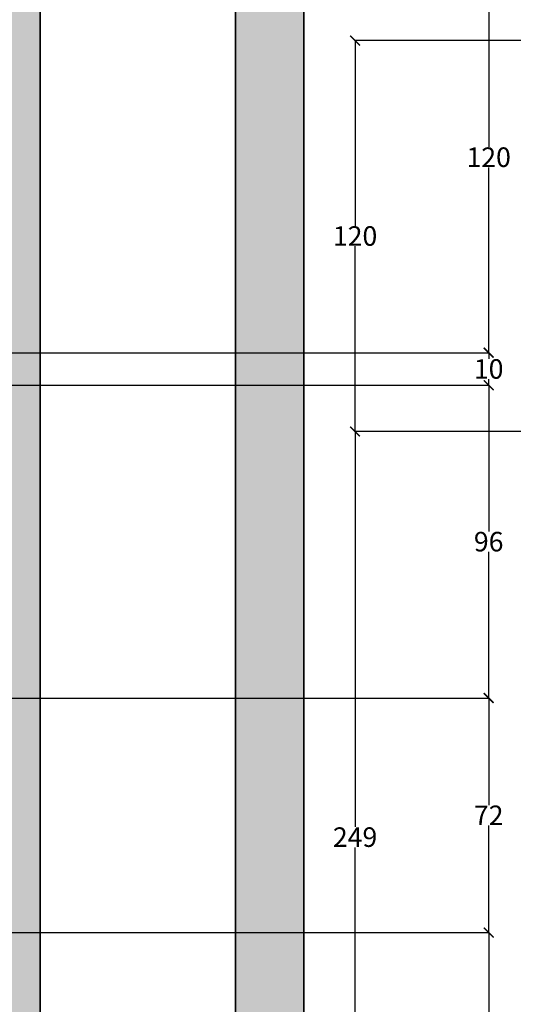
# Model space of a CAD drawing. Units: inches. Extents: x 925 to 2834, y 111 to 1355.
# Tile 22 of 25: x 1844 to 1996, y 882 to 1184. Entities that reach past the tile are written whole.
import ezdxf

# ---------------------------------------------------------------- set-up
doc = ezdxf.new("R2010")
doc.units = ezdxf.units.IN
doc.header["$MEASUREMENT"] = 0
for name, color, linetype, lineweight in [('A-ANNO-DIMS', 2, 'Continuous', 18), ('A-ANNO-TTLB', 7, 'Continuous', 35), ('A-FLOR-PATT', 252, 'Continuous', 13)]:
    doc.layers.add(name, color=color, linetype=linetype, lineweight=lineweight)
doc.styles.get("Standard").update_dxf_attribs({"font": 'arial.ttf'})
doc.dimstyles.get("Standard").update_dxf_attribs({"dimtxt": 6, "dimasz": 3, "dimexe": 0.18, "dimexo": 0.0625, "dimgap": 0.09, "dimtad": 0, "dimtih": 1, "dimtoh": 1, "dimdec": 1, "dimzin": 0, "dimdsep": 46, "dimlunit": 3, "dimtxsty": 'Standard', "dimblk": 'ARCHTICK', "dimcen": 0.09, "dimadec": 0, "dimazin": 0, "dimtfac": 1, "dimtdec": 1, "dimtofl": 0, "dimtmove": 0, "dimatfit": 3, "dimfxl": 1, "dimtolj": 1, "dimtzin": 0, "dimarcsym": 0})

# ---------------------------------------------------------------- blocks, each defined once
blk = doc.blocks.new('_ArchTick')
at = {"color": 0, "linetype": 'ByBlock', "const_width": 0.15}
blk.add_lwpolyline([(-0.5, -0.5), (0.5, 0.5)], dxfattribs=at)
blk = doc.blocks.new('*D47')
at = {"layer": 'A-ANNO-DIMS', "color": 0, "lineweight": -2, "transparency": 16777216}
for p, q in [((1708.78, 903.59), (1988.62, 903.59)), ((1988.44, 903.59), (1988.44, 869.23)), ((1988.44, 828.59), (1988.44, 862.95)), ((1708.78, 828.59), (1988.62, 828.59))]:
    blk.add_line(p, q, dxfattribs=at)
at = {"layer": 'Defpoints', "color": 0, "transparency": 16777216}
for p in [(1708.71, 903.59), (1988.44, 903.59), (1708.71, 828.59)]:
    blk.add_point(p, dxfattribs=at)
at = {"layer": 'A-ANNO-DIMS', "color": 0, "lineweight": -2, "transparency": 16777216, "xscale": 3, "yscale": 3, "zscale": 3}
for p, rotation in [((1988.44, 903.59), 90), ((1988.44, 828.59), 270)]:
    blk.add_blockref('_ArchTick', p, dxfattribs=dict(at, rotation=rotation))
at = {"layer": 'A-ANNO-DIMS', "color": 0, "transparency": 16777216, "insert": (1988.44, 866.09), "char_height": 6, "attachment_point": 5}
blk.add_mtext('\\A1;75', dxfattribs=at)
blk = doc.blocks.new('*D48')
at = {"layer": 'A-ANNO-DIMS', "color": 0, "lineweight": -2, "transparency": 16777216}
for p, q in [((1708.78, 975.59), (1988.62, 975.59)), ((1988.44, 975.59), (1988.44, 942.69)), ((1988.44, 903.59), (1988.44, 936.49)), ((1708.78, 903.59), (1988.62, 903.59))]:
    blk.add_line(p, q, dxfattribs=at)
at = {"layer": 'Defpoints', "color": 0, "transparency": 16777216}
for p in [(1708.71, 975.59), (1988.44, 975.59), (1708.71, 903.59)]:
    blk.add_point(p, dxfattribs=at)
at = {"layer": 'A-ANNO-DIMS', "color": 0, "lineweight": -2, "transparency": 16777216, "xscale": 3, "yscale": 3, "zscale": 3}
for p, rotation in [((1988.44, 975.59), 90), ((1988.44, 903.59), 270)]:
    blk.add_blockref('_ArchTick', p, dxfattribs=dict(at, rotation=rotation))
at = {"layer": 'A-ANNO-DIMS', "color": 0, "transparency": 16777216, "insert": (1988.44, 939.59), "char_height": 6, "attachment_point": 5}
blk.add_mtext('\\A1;72', dxfattribs=at)
blk = doc.blocks.new('*D49')
at = {"layer": 'A-ANNO-DIMS', "color": 0, "lineweight": -2, "transparency": 16777216}
for p, q in [((1708.78, 1071.59), (1988.62, 1071.59)), ((1988.44, 1071.59), (1988.44, 1026.74)), ((1988.44, 975.59), (1988.44, 1020.44)), ((1708.78, 975.59), (1988.62, 975.59))]:
    blk.add_line(p, q, dxfattribs=at)
at = {"layer": 'Defpoints', "color": 0, "transparency": 16777216}
for p in [(1708.71, 1071.59), (1988.44, 1071.59), (1708.71, 975.59)]:
    blk.add_point(p, dxfattribs=at)
at = {"layer": 'A-ANNO-DIMS', "color": 0, "lineweight": -2, "transparency": 16777216, "xscale": 3, "yscale": 3, "zscale": 3}
for p, rotation in [((1988.44, 1071.59), 90), ((1988.44, 975.59), 270)]:
    blk.add_blockref('_ArchTick', p, dxfattribs=dict(at, rotation=rotation))
at = {"layer": 'A-ANNO-DIMS', "color": 0, "transparency": 16777216, "insert": (1988.44, 1023.59), "char_height": 6, "attachment_point": 5}
blk.add_mtext('\\A1;96', dxfattribs=at)
blk = doc.blocks.new('*D50')
at = {"layer": 'A-ANNO-DIMS', "color": 0, "lineweight": -2, "transparency": 16777216}
for p, q in [((1718.78, 1081.59), (1988.62, 1081.59)), ((1988.44, 1081.59), (1988.44, 1079.74)), ((1988.44, 1071.59), (1988.44, 1073.44)), ((1708.78, 1071.59), (1988.62, 1071.59))]:
    blk.add_line(p, q, dxfattribs=at)
at = {"layer": 'Defpoints', "color": 0, "transparency": 16777216}
for p in [(1718.71, 1081.59), (1988.44, 1081.59), (1708.71, 1071.59)]:
    blk.add_point(p, dxfattribs=at)
at = {"layer": 'A-ANNO-DIMS', "color": 0, "lineweight": -2, "transparency": 16777216, "xscale": 3, "yscale": 3, "zscale": 3}
for p, rotation in [((1988.44, 1081.59), 90), ((1988.44, 1071.59), 270)]:
    blk.add_blockref('_ArchTick', p, dxfattribs=dict(at, rotation=rotation))
at = {"layer": 'A-ANNO-DIMS', "color": 0, "transparency": 16777216, "insert": (1988.44, 1076.59), "char_height": 6, "attachment_point": 5}
blk.add_mtext('\\A1;10', dxfattribs=at)
blk = doc.blocks.new('*D51')
at = {"layer": 'A-ANNO-DIMS', "color": 0, "lineweight": -2, "transparency": 16777216}
for p, q in [((1838.78, 1201.59), (1988.62, 1201.59)), ((1988.44, 1201.59), (1988.44, 1144.74)), ((1988.44, 1081.59), (1988.44, 1138.44)), ((1718.78, 1081.59), (1988.62, 1081.59))]:
    blk.add_line(p, q, dxfattribs=at)
at = {"layer": 'Defpoints', "color": 0, "transparency": 16777216}
for p in [(1838.71, 1201.59), (1988.44, 1201.59), (1718.71, 1081.59)]:
    blk.add_point(p, dxfattribs=at)
at = {"layer": 'A-ANNO-DIMS', "color": 0, "lineweight": -2, "transparency": 16777216, "xscale": 3, "yscale": 3, "zscale": 3}
for p, rotation in [((1988.44, 1201.59), 90), ((1988.44, 1081.59), 270)]:
    blk.add_blockref('_ArchTick', p, dxfattribs=dict(at, rotation=rotation))
at = {"layer": 'A-ANNO-DIMS', "color": 0, "transparency": 16777216, "insert": (1988.44, 1141.59), "char_height": 6, "attachment_point": 5}
blk.add_mtext('\\A1;120', dxfattribs=at)
blk = doc.blocks.new('*D79')
at = {"layer": 'A-ANNO-DIMS', "color": 0, "lineweight": -2, "transparency": 16777216}
for p, q in [((2143.61, 1057.4), (1947.23, 1057.4)), ((1947.41, 1057.4), (1947.41, 936.05)), ((1947.41, 808.4), (1947.41, 929.74)), ((2124.2, 808.4), (1947.23, 808.4))]:
    blk.add_line(p, q, dxfattribs=at)
at = {"layer": 'Defpoints', "color": 0, "transparency": 16777216}
for p in [(1947.41, 1057.4), (2143.68, 1057.4), (2124.26, 808.4)]:
    blk.add_point(p, dxfattribs=at)
at = {"layer": 'A-ANNO-DIMS', "color": 0, "lineweight": -2, "transparency": 16777216, "xscale": 3, "yscale": 3, "zscale": 3}
for p, rotation in [((1947.41, 1057.4), 90), ((1947.41, 808.4), 270)]:
    blk.add_blockref('_ArchTick', p, dxfattribs=dict(at, rotation=rotation))
at = {"layer": 'A-ANNO-DIMS', "color": 0, "transparency": 16777216, "insert": (1947.41, 932.9), "char_height": 6, "attachment_point": 5}
blk.add_mtext('\\A1;249', dxfattribs=at)
blk = doc.blocks.new('*D80')
at = {"layer": 'A-ANNO-DIMS', "color": 0, "lineweight": -2, "transparency": 16777216}
for p, q in [((2008.7, 1177.4), (1947.23, 1177.4)), ((1947.41, 1177.4), (1947.41, 1120.55)), ((1947.41, 1057.4), (1947.41, 1114.24)), ((2143.61, 1057.4), (1947.23, 1057.4))]:
    blk.add_line(p, q, dxfattribs=at)
at = {"layer": 'Defpoints', "color": 0, "transparency": 16777216}
for p in [(1947.41, 1177.4), (2008.76, 1177.4), (2143.68, 1057.4)]:
    blk.add_point(p, dxfattribs=at)
at = {"layer": 'A-ANNO-DIMS', "color": 0, "lineweight": -2, "transparency": 16777216, "xscale": 3, "yscale": 3, "zscale": 3}
for p, rotation in [((1947.41, 1177.4), 90), ((1947.41, 1057.4), 270)]:
    blk.add_blockref('_ArchTick', p, dxfattribs=dict(at, rotation=rotation))
at = {"layer": 'A-ANNO-DIMS', "color": 0, "transparency": 16777216, "insert": (1947.41, 1117.4), "char_height": 6, "attachment_point": 5}
blk.add_mtext('\\A1;120', dxfattribs=at)

msp = doc.modelspace()

# ---------------------------------------------------------------- hatches: boundary and pattern name
at = {"layer": 'A-FLOR-PATT', "transparency": 33554605}
h = msp.add_hatch(color=256, dxfattribs=at)
h.dxf.hatch_style = 1
h.paths.add_polyline_path([(1931.688, 1294.5638), (991.7375, 1294.5638), (991.7375, 172.1134), (1931.688, 172.1134)])
h.paths.add_polyline_path([(1910.7128, 1273.5886), (1910.7128, 193.0886), (1012.7128, 193.0886), (1012.7128, 1273.5886)], flags=16)
h.paths.add_polyline_path([(1850.7128, 1213.5886), (1850.7128, 253.0886), (1072.7128, 253.0886), (1072.7128, 1213.5886)], flags=0)
h.paths.add_polyline_path([(1838.7128, 1201.5886), (1838.7128, 265.0886), (1084.7128, 265.0886), (1084.7128, 530.5886), (1084.7128, 1201.5886)], flags=0)
h.paths.add_polyline_path([(1547.6758, 1155.7396), (1547.6758, 1119.115), (1513.0687, 1119.115), (1513.0687, 1155.7396)], flags=0)
h.paths.add_polyline_path([(1600.1067, 1154.9439), (1634.7139, 1154.9439), (1634.7139, 1119.115), (1600.1067, 1119.115)], flags=0)
h.paths.add_polyline_path([(1505.2502, 1144.5358), (1505.2502, 1119.115), (1470.643, 1119.115), (1470.643, 1144.5358)], flags=0)
h.paths.add_polyline_path([(1559.1357, 1141.0962), (1593.7428, 1141.0962), (1593.7428, 1119.115), (1559.1357, 1119.115)], flags=0)
h.paths.add_polyline_path([(1462.8966, 1154.9439), (1462.8966, 1119.115), (1428.2895, 1119.115), (1428.2895, 1154.9439)], flags=0)
h.paths.add_polyline_path([(1642.4603, 1144.5358), (1677.0675, 1144.5358), (1677.0675, 1119.115), (1642.4603, 1119.115)], flags=0)
h.paths.add_polyline_path([(1422.3508, 1141.0962), (1422.3508, 1119.115), (1387.7436, 1119.115), (1387.7436, 1141.0962)], flags=0)
h.paths.add_polyline_path([(1684.8859, 1155.7396), (1719.4931, 1155.7396), (1719.4931, 1119.115), (1684.8859, 1119.115)], flags=0)
h.paths.add_polyline_path([(1718.7128, 1081.5886), (1718.7128, 1050.1249), (1715.7128, 1050.1249), (1715.7128, 1026.1249), (1715.7128, 1002.1249), (1718.7128, 1002.1249), (1730.7128, 1002.1249), (1730.7128, 998.1249), (1730.7128, 990.1249), (1730.7128, 986.1249), (1718.7128, 986.1249), (1718.7128, 893.5886), (1715.3735, 893.5886), (1715.3735, 891.5886), (1713.3735, 891.5886, 0.41421356), (1677.3735, 855.5886), (1713.3735, 855.5886), (1713.3735, 853.5886), (1715.3735, 853.5886), (1715.3735, 851.5886), (1718.7128, 851.5886), (1718.7128, 821.5865), (1734.4655, 821.5865), (1734.3735, 819.5886, -0.41421356), (1712.4415, 793.5886), (1712.4415, 791.5886), (1718.7128, 791.5886), (1718.7128, 717.5886), (1718.7128, 669.5886), (1732.7128, 669.5886), (1732.7128, 665.5886), (1732.7128, 641.5886), (1732.7128, 634.5886), (1732.7128, 610.5886), (1732.7128, 603.5886), (1718.7128, 603.5886), (1718.7128, 385.0886), (1434.2128, 385.0886), (1434.2128, 530.5886), (1410.2128, 530.5886), (1408.2128, 530.5886), (1408.2128, 532.5886, 0.41421356), (1372.2128, 568.5886), (1372.2128, 532.5886), (1370.2128, 532.5886), (1370.2128, 530.5886), (1368.2128, 530.5886), (1282.2128, 530.5886), (1210.2128, 530.5886), (1200.2128, 530.5886), (1200.2128, 542.1915), (1183.2307, 542.1915), (1183.2307, 546.1915), (1200.2128, 546.1915), (1200.2128, 572.1915), (1183.2307, 572.1915), (1183.2307, 576.1915), (1200.2128, 576.1915), (1200.2128, 727.5886), (1210.2128, 727.5886), (1234.2128, 727.5886), (1259.7128, 727.5886), (1259.7128, 775.5886), (1259.7128, 799.5886), (1259.7128, 847.5886), (1259.7128, 993.5872), (1259.7128, 1065.5872), (1259.7128, 1071.5886), (1219.6318, 1071.5886), (1219.6318, 1081.5886), (1084.7128, 1081.5886), (1084.7128, 1119.115), (1256.8974, 1119.115), (1256.8974, 1154.9439), (1291.5046, 1154.9439), (1291.5046, 1119.115), (1256.8974, 1119.115), (1256.6723, 1081.5886), (1293.7128, 1081.5886), (1341.7128, 1081.5886), (1341.7128, 1093.5886), (1347.7128, 1093.5886), (1371.7128, 1093.5886), (1377.7128, 1093.5886), (1377.7128, 1081.5886), (1668.7128, 1081.5886), (1668.7128, 1117.5886), (1675.7128, 1117.5886), (1711.7128, 1117.5886), (1718.7128, 1117.5886)], flags=0)
h.paths.add_polyline_path([(1376.2838, 1155.7396), (1376.2838, 1119.115), (1341.6766, 1119.115), (1341.6766, 1155.7396)], flags=0)
h.paths.add_polyline_path([(1341.7128, 1076.0886), (1293.7128, 1076.0886), (1293.7128, 1071.5886), (1269.7128, 1071.5886), (1269.7128, 1065.5872), (1266.7128, 1065.5872), (1266.7128, 1029.5872), (1265.7128, 1029.5872), (1265.7128, 993.5872), (1269.7128, 993.5872), (1269.7128, 903.5886), (1269.7128, 893.5886), (1269.7128, 847.5886), (1265.2128, 847.5886), (1265.2128, 799.5886), (1269.7128, 799.5886), (1269.7128, 775.5886), (1265.2128, 775.5886), (1265.2128, 727.5886), (1269.7128, 727.5886), (1444.2128, 727.5886), (1444.2128, 717.5886), (1234.2128, 717.5886), (1234.2128, 722.0886), (1210.2128, 722.0886), (1210.2128, 717.5886), (1210.2128, 540.5886), (1210.2128, 536.0886), (1282.2128, 536.0886), (1282.2128, 535.0886), (1210.2128, 535.0886), (1210.2128, 540.5886), (1210.2128, 717.5886), (1210.2128, 723.0886), (1234.2128, 723.0886), (1234.2128, 717.5886), (1444.2128, 717.5886), (1444.2128, 727.5886), (1269.7128, 727.5886), (1264.2128, 727.5886), (1264.2128, 775.5886), (1269.7128, 775.5886), (1269.7128, 799.5886), (1264.2128, 799.5886), (1264.2128, 847.5886), (1269.7128, 847.5886), (1269.7128, 893.5886), (1269.7128, 903.5886), (1269.7128, 993.5872), (1264.7128, 993.5872), (1264.7128, 1029.5872), (1265.7128, 1029.5872), (1265.7128, 1065.5872), (1269.7128, 1065.5872), (1269.7128, 1071.5886), (1293.7128, 1071.5886), (1293.7128, 1077.0886), (1341.7128, 1077.0886)], flags=0)
h.paths.add_polyline_path([(1730.9529, 1141.0962), (1765.5601, 1141.0962), (1765.5601, 1119.115), (1730.9529, 1119.115)], flags=0)
h.paths.add_polyline_path([(1333.8582, 1144.5358), (1333.8582, 1119.115), (1299.251, 1119.115), (1299.251, 1144.5358)], flags=0)
h.paths.add_polyline_path([(1592.7128, 968.5886), (1596.0342, 968.5886), (1602.7128, 968.5886), (1708.7128, 968.5886), (1708.7128, 903.5886), (1602.7128, 903.5886), (1602.7128, 938.5886), (1592.7128, 938.5886), (1592.7128, 903.5886), (1451.7128, 903.5886), (1451.7128, 893.5886), (1511.7128, 893.5886), (1511.7128, 881.5886), (1515.2128, 881.5886), (1518.7128, 881.5886), (1518.7128, 893.5886), (1592.7128, 893.5886), (1592.7128, 799.5886), (1518.7128, 799.5886), (1518.7128, 857.5886), (1511.7128, 857.5886), (1511.7128, 799.5886), (1511.7128, 772.0886), (1521.7128, 772.0886), (1521.7128, 792.5886), (1592.7128, 792.5886), (1592.7128, 727.5886), (1521.7128, 727.5886), (1521.7128, 748.0886), (1511.7128, 748.0886), (1511.7128, 717.5886), (1708.7128, 717.5886), (1714.2128, 717.5886), (1714.2128, 669.5886), (1708.7128, 669.5886), (1708.7128, 641.5886), (1492.2128, 641.5886), (1492.2128, 631.5886), (1621.2128, 631.5886), (1621.2128, 443.0886), (1625.7128, 443.0886), (1625.7128, 503.0886), (1625.7128, 507.5886), (1625.7128, 631.5886), (1708.7128, 631.5886), (1708.7128, 507.5886), (1655.7128, 507.5886), (1655.7128, 503.0886), (1708.7128, 503.0886), (1708.7128, 395.0886), (1625.7128, 395.0886), (1625.7128, 419.0886), (1621.2128, 419.0886), (1621.2128, 395.0886), (1482.2128, 395.0886), (1482.2128, 385.0886), (1434.2128, 385.0886), (1434.2128, 433.0886), (1444.2128, 433.0886), (1444.2128, 631.5886), (1450.2128, 631.5886), (1450.2128, 634.91), (1452.2128, 634.91), (1452.2128, 669.5886), (1454.2128, 669.5886, -0.40021217), (1490.1712, 635.3173), (1492.2128, 635.3173), (1492.2128, 641.5886), (1564.7128, 641.5886), (1564.7128, 677.5886), (1672.7128, 677.5886), (1672.7128, 681.5886), (1564.7128, 681.5886), (1564.7128, 717.5886), (1511.7128, 717.5886), (1511.7128, 748.0886), (1511.7128, 772.0886), (1511.7128, 799.5886), (1511.7128, 857.5886), (1511.8913, 857.5886), (1511.8913, 859.5886), (1515.6201, 859.5886, 0.41421356), (1537.552, 879.5886), (1513.552, 879.5886), (1511.8913, 879.5886), (1511.8913, 881.5886), (1511.7128, 881.5886), (1511.7128, 893.5886), (1451.7128, 893.5886), (1451.7128, 903.5886), (1592.7128, 903.5886), (1592.7128, 938.5886), (1592.7128, 940.5886), (1596.4415, 940.5886, 0.41421356), (1618.3735, 966.5886), (1594.3735, 966.5886), (1592.7128, 966.5886)], flags=0)
h.paths.add_polyline_path([(1377.7128, 903.5886), (1377.7128, 893.5886), (1305.7128, 893.5886), (1305.7128, 903.5886)], flags=0)
h.paths.add_polyline_path([(1708.7128, 821.5886), (1712.0342, 821.5886), (1712.0342, 819.5886), (1710.3735, 819.5886), (1708.7128, 819.5886)], flags=0)
h.paths.add_polyline_path([(1576.7128, 695.1992), (1575.5896, 693.6649), (1575.9687, 694.6994), (1575.4438, 695.1992), (1575.9687, 695.699), (1575.5896, 696.7335)], flags=0)
h.paths.add_polyline_path([(1565.9817, 662.3134), (1565.4568, 661.8136), (1565.8359, 660.7791), (1564.7128, 662.3134), (1565.8359, 663.8477), (1565.4568, 662.8132)], flags=0)
h.paths.add_polyline_path([(1444.2128, 433.0886), (1444.2128, 395.0886), (1482.2128, 395.0886), (1482.2128, 389.0886), (1438.2128, 389.0886), (1438.2128, 391.8608), (1438.2128, 433.0886)], flags=0)
h.paths.add_polyline_path([(1410.2128, 506.5886), (1410.2128, 289.0886), (1108.7128, 289.0886), (1108.7128, 506.5886)], flags=0)
h.paths.add_polyline_path([(1612.3153, 838.3016), (1680.4151, 838.3016), (1680.4151, 851.3131), (1612.3153, 851.3131)], flags=8)
h.paths.add_polyline_path([(1208.3174, 395.0436), (1282.1017, 395.0436), (1282.1017, 408.0552), (1208.3174, 408.0552)], flags=8)
h.paths.add_polyline_path([(1291.8049, 598.7427), (1369.8017, 598.7427), (1369.8017, 611.7542), (1291.8049, 611.7542)], flags=8)
h.paths.add_polyline_path([(1119.679, 917.3022), (1191.0817, 917.3022), (1191.0817, 930.3137), (1119.679, 930.3137)], flags=8)
h.paths.add_polyline_path([(1332.2261, 815.9808), (1410.2258, 815.9808), (1410.2258, 829.001), (1332.2261, 829.001)], flags=8)
h.paths.add_polyline_path([(1390.9013, 955.8158), (1475.4981, 955.8158), (1475.4981, 968.8273), (1390.9013, 968.8273)], flags=8)
h.paths.add_polyline_path([(1620.3436, 998.9325), (1688.4434, 998.9325), (1688.4434, 1011.944), (1620.3436, 1011.944)], flags=8)
h.paths.add_polyline_path([(1620.3436, 914.1039), (1691.7405, 914.1039), (1691.7405, 927.1155), (1620.3436, 927.1155)], flags=8)
h.paths.add_polyline_path([(1521.4542, 816.005), (1589.5569, 816.005), (1589.5569, 829.0253), (1521.4542, 829.0253)], flags=8)
h.paths.add_polyline_path([(1528.524, 740.3497), (1602.3082, 740.3497), (1602.3082, 753.3613), (1528.524, 753.3613)], flags=8)
h.paths.add_polyline_path([(1627.6094, 762.6128), (1702.3091, 762.6128), (1702.3091, 775.6244), (1627.6094, 775.6244)], flags=8)
h.paths.add_polyline_path([(1610.5442, 657.2751), (1684.3284, 657.2751), (1684.3284, 670.2867), (1610.5442, 670.2867)], flags=8)
h.paths.add_polyline_path([(1636.6983, 519.472), (1711.3981, 519.472), (1711.3981, 532.4835), (1636.6983, 532.4835)], flags=8)
h.paths.add_polyline_path([(1616.8577, 424.8539), (1694.8545, 424.8539), (1694.8545, 437.8654), (1616.8577, 437.8654)], flags=8)
h.paths.add_polyline_path([(1506.1456, 460.8838), (1579.9299, 460.8838), (1579.9299, 473.8953), (1506.1456, 473.8953)], flags=8)
h.paths.add_polyline_path([(1624.6119, 784.6011), (1696.9185, 784.6011), (1696.9185, 797.7864), (1624.6119, 797.7864)], flags=8)
h.paths.add_polyline_path([(1606.3732, 854.2194), (1683.3039, 854.2194), (1683.3039, 867.4048), (1606.3732, 867.4048)], flags=8)
h.paths.add_polyline_path([(1127.8008, 940.3581), (1165.1637, 940.3581), (1165.1637, 953.5348), (1127.8008, 953.5348)], flags=8)
h.paths.add_polyline_path([(1620.8657, 1019.4968), (1677.3447, 1019.4968), (1677.3447, 1032.6735), (1620.8657, 1032.6735)], flags=8)
h.paths.add_polyline_path([(1620.8643, 930.1821), (1703.0564, 930.1821), (1703.0564, 943.3675), (1620.8643, 943.3675)], flags=8)
h.paths.add_polyline_path([(1324.5702, 836.8338), (1408.0892, 836.8338), (1408.0892, 850.0191), (1324.5702, 850.0191)], flags=8)
h.paths.add_polyline_path([(1281.6584, 622.8885), (1383.6213, 622.8885), (1383.6213, 636.0739), (1281.6584, 636.0739)], flags=8)
h.paths.add_polyline_path([(1210.6721, 416.7893), (1269.1299, 416.7893), (1269.1299, 429.9747), (1210.6721, 429.9747)], flags=8)
h.paths.add_polyline_path([(1507.8264, 477.4836), (1586.7329, 477.4836), (1586.7329, 490.669), (1507.8264, 490.669)], flags=8)
h.paths.add_polyline_path([(1643.6238, 443.8135), (1696.6696, 443.8135), (1696.6696, 456.5643), (1643.6238, 456.5643)], flags=8)
h.paths.add_polyline_path([(1647.2466, 540.5638), (1693.1825, 540.5638), (1693.1825, 553.7491), (1647.2466, 553.7491)], flags=8)
h.paths.add_polyline_path([(1626.0633, 668.5064), (1673.3174, 668.5064), (1673.3174, 681.6831), (1626.0633, 681.6831)], flags=8)
h.paths.add_polyline_path([(1538.2915, 830.7872), (1567.5942, 830.7872), (1567.5942, 843.5293), (1538.2915, 843.5293)], flags=8)
h.paths.add_polyline_path([(1530.9338, 754.0477), (1559.576, 754.0477), (1559.576, 766.7898), (1530.9338, 766.7898)], flags=8)
h.paths.add_polyline_path([(1351.2461, 979.2309), (1513.8919, 979.2309), (1513.8919, 992.4076), (1351.2461, 992.4076)], flags=8)
at = {"layer": 'A-FLOR-PATT'}
h = msp.add_hatch(color=256, dxfattribs=at)
h.dxf.hatch_style = 1
h.paths.add_polyline_path([(1850.7128, 1213.5886), (1072.7128, 1213.5886), (1072.7128, 253.0886), (1850.7128, 253.0886)])
h.paths.add_polyline_path([(1084.7128, 1201.5886), (1838.7128, 1201.5886), (1838.7128, 265.0886), (1084.7128, 265.0886)], flags=16)
h.paths.add_polyline_path([(1183.2307, 576.1915), (1200.2128, 576.1915), (1200.2128, 727.5886), (1210.2128, 727.5886), (1234.2128, 727.5886), (1259.7128, 727.5886), (1259.7128, 775.5886), (1259.7128, 799.5886), (1259.7128, 847.5886), (1259.7128, 993.5872), (1259.7128, 1065.5872), (1259.7128, 1071.5886), (1219.6318, 1071.5886), (1219.6318, 1081.5886), (1293.7128, 1081.5886), (1341.7128, 1081.5886), (1341.7128, 1093.5886), (1347.7128, 1093.5886), (1347.7128, 1081.5886), (1371.7128, 1081.5886), (1371.7128, 1093.5886), (1377.7128, 1093.5886), (1377.7128, 1081.5886), (1668.7128, 1081.5886), (1668.7128, 1117.5886), (1675.7128, 1117.5886), (1675.7128, 1081.5886), (1711.7128, 1081.5886), (1711.7128, 1117.5886), (1718.7128, 1117.5886), (1718.7128, 1081.5886), (1718.7128, 1050.1249), (1715.7128, 1050.1249), (1715.7128, 1026.1249), (1715.7128, 1002.1249), (1718.7128, 1002.1249), (1730.7128, 1002.1249), (1730.7128, 998.1249), (1730.7128, 990.1249), (1730.7128, 986.1249), (1718.7128, 986.1249), (1718.7128, 893.5886), (1715.3735, 893.5886), (1715.3735, 891.5886), (1713.3735, 891.5886, 0.41421356), (1677.3735, 855.5886), (1713.3735, 855.5886), (1713.3735, 853.5886), (1715.3735, 853.5886), (1715.3735, 851.5886), (1718.7128, 851.5886), (1718.7128, 821.5865), (1734.4655, 821.5865), (1734.3735, 819.5886, -0.41421356), (1712.4415, 793.5886), (1712.4415, 791.5886), (1718.7128, 791.5886), (1718.7128, 717.5886), (1718.7128, 669.5886), (1732.7128, 669.5886), (1732.7128, 665.5886), (1732.7128, 641.5886), (1732.7128, 634.5886), (1732.7128, 610.5886), (1732.7128, 603.5886), (1718.7128, 603.5886), (1718.7128, 385.0886), (1434.2128, 385.0886), (1434.2128, 433.0886), (1434.2128, 530.5886), (1410.2128, 530.5886), (1408.2128, 530.5886), (1408.2128, 532.5886, 0.41421356), (1372.2128, 568.5886), (1372.2128, 532.5886), (1370.2128, 532.5886), (1370.2128, 530.5886), (1368.2128, 530.5886), (1282.2128, 530.5886), (1210.2128, 530.5886), (1200.2128, 530.5886), (1200.2128, 542.1915), (1183.2307, 542.1915), (1183.2307, 546.1915), (1200.2128, 546.1915), (1200.2128, 572.1915), (1183.2307, 572.1915)], flags=0)
h.paths.add_polyline_path([(1210.2128, 717.5886), (1210.2128, 723.0886), (1234.2128, 723.0886), (1234.2128, 717.5886), (1444.2128, 717.5886), (1444.2128, 727.5886), (1269.7128, 727.5886), (1264.2128, 727.5886), (1264.2128, 775.5886), (1269.7128, 775.5886), (1269.7128, 799.5886), (1264.2128, 799.5886), (1264.2128, 847.5886), (1269.7128, 847.5886), (1269.7128, 893.5886), (1269.7128, 903.5886), (1269.7128, 993.5872), (1264.7128, 993.5872), (1264.7128, 1029.5872), (1265.7128, 1029.5872), (1265.7128, 1065.5872), (1269.7128, 1065.5872), (1269.7128, 1071.5886), (1293.7128, 1071.5886), (1293.7128, 1077.0886), (1341.7128, 1077.0886), (1341.7128, 1076.0886), (1293.7128, 1076.0886), (1293.7128, 1071.5886), (1269.7128, 1071.5886), (1269.7128, 1065.5872), (1266.7128, 1065.5872), (1266.7128, 1029.5872), (1265.7128, 1029.5872), (1265.7128, 993.5872), (1269.7128, 993.5872), (1269.7128, 903.5886), (1269.7128, 893.5886), (1269.7128, 847.5886), (1265.2128, 847.5886), (1265.2128, 799.5886), (1269.7128, 799.5886), (1269.7128, 775.5886), (1265.2128, 775.5886), (1265.2128, 727.5886), (1269.7128, 727.5886), (1444.2128, 727.5886), (1444.2128, 717.5886), (1234.2128, 717.5886), (1234.2128, 722.0886), (1210.2128, 722.0886), (1210.2128, 717.5886), (1210.2128, 540.5886), (1210.2128, 536.0886), (1282.2128, 536.0886), (1282.2128, 535.0886), (1210.2128, 535.0886), (1210.2128, 540.5886)], flags=0)
h.paths.add_polyline_path([(1450.2128, 634.91), (1452.2128, 634.91), (1452.2128, 669.5886), (1454.2128, 669.5886, -0.40021217), (1490.1712, 635.3173), (1492.2128, 635.3173), (1492.2128, 641.5886), (1564.7128, 641.5886), (1564.7128, 677.5886), (1672.7128, 677.5886), (1672.7128, 681.5886), (1564.7128, 681.5886), (1564.7128, 717.5886), (1511.7128, 717.5886), (1511.7128, 748.0886), (1511.7128, 772.0886), (1511.7128, 799.5886), (1511.7128, 857.5886), (1511.8913, 857.5886), (1511.8913, 859.5886), (1515.6201, 859.5886, 0.41421356), (1537.552, 879.5886), (1513.552, 879.5886), (1511.8913, 879.5886), (1511.8913, 881.5886), (1511.7128, 881.5886), (1511.7128, 893.5886), (1451.7128, 893.5886), (1451.7128, 903.5886), (1592.7128, 903.5886), (1592.7128, 938.5886), (1592.7128, 940.5886), (1596.4415, 940.5886, 0.41421356), (1618.3735, 966.5886), (1594.3735, 966.5886), (1592.7128, 966.5886), (1592.7128, 968.5886), (1596.0342, 968.5886), (1602.7128, 968.5886), (1708.7128, 968.5886), (1708.7128, 903.5886), (1602.7128, 903.5886), (1602.7128, 938.5886), (1592.7128, 938.5886), (1592.7128, 903.5886), (1451.7128, 903.5886), (1451.7128, 893.5886), (1511.7128, 893.5886), (1511.7128, 881.5886), (1518.7128, 881.5886), (1518.7128, 893.5886), (1592.7128, 893.5886), (1592.7128, 799.5886), (1518.7128, 799.5886), (1518.7128, 857.5886), (1511.7128, 857.5886), (1511.7128, 799.5886), (1511.7128, 772.0886), (1521.7128, 772.0886), (1521.7128, 792.5886), (1592.7128, 792.5886), (1592.7128, 727.5886), (1521.7128, 727.5886), (1521.7128, 748.0886), (1511.7128, 748.0886), (1511.7128, 717.5886), (1708.7128, 717.5886), (1714.2128, 717.5886), (1714.2128, 669.5886), (1708.7128, 669.5886), (1708.7128, 641.5886), (1492.2128, 641.5886), (1492.2128, 631.5886), (1621.2128, 631.5886), (1621.2128, 443.0886), (1625.7128, 443.0886), (1625.7128, 503.0886), (1625.7128, 507.5886), (1625.7128, 631.5886), (1708.7128, 631.5886), (1708.7128, 507.5886), (1655.7128, 507.5886), (1655.7128, 503.0886), (1708.7128, 503.0886), (1708.7128, 395.0886), (1625.7128, 395.0886), (1625.7128, 419.0886), (1621.2128, 419.0886), (1621.2128, 395.0886), (1482.2128, 395.0886), (1482.2128, 389.0886), (1438.2128, 389.0886), (1438.2128, 391.8608), (1438.2128, 433.0886), (1444.2128, 433.0886), (1444.2128, 631.5886), (1450.2128, 631.5886)], flags=0)
h.paths.add_polyline_path([(1444.2128, 433.0886), (1444.2128, 395.0886), (1482.2128, 395.0886), (1482.2128, 391.0886), (1440.2128, 391.0886), (1440.2128, 391.8608), (1440.2128, 433.0886)], flags=0)
h.paths.add_polyline_path([(1305.7128, 893.5886), (1305.7128, 903.5886), (1377.7128, 903.5886), (1377.7128, 893.5886)], flags=0)
h.paths.add_polyline_path([(1564.7128, 662.3134), (1565.8359, 663.8477), (1565.4568, 662.8132), (1565.9817, 662.3134), (1565.4568, 661.8136), (1565.8359, 660.7791)], flags=0)
h.paths.add_polyline_path([(1575.4438, 695.1992), (1575.9687, 695.699), (1575.5896, 696.7335), (1576.7128, 695.1992), (1575.5896, 693.6649), (1575.9687, 694.6994)], flags=0)
h.paths.add_polyline_path([(1708.7128, 821.5886), (1712.0342, 821.5886), (1712.0342, 819.5886), (1710.3735, 819.5886), (1708.7128, 819.5886)], flags=0)

# ---------------------------------------------------------------- linework, layer by layer
at = {"layer": 'A-ANNO-TTLB'}
for points in [[(991.7375, 172.1134), (1931.688, 172.1134), (1931.688, 1294.5638), (991.7375, 1294.5638)], [(1012.7128, 193.0886), (1910.7128, 193.0886), (1910.7128, 1273.5886), (1012.7128, 1273.5886)], [(1072.7128, 253.0886), (1850.7128, 253.0886), (1850.7128, 1213.5886), (1072.7128, 1213.5886)]]:
    msp.add_lwpolyline(points, close=True, dxfattribs=at)

# ---------------------------------------------------------------- dimensions: what is measured, and where the dimension line sits
at = {"layer": 'A-ANNO-DIMS'}
for base, p1, p2, picture, middle in [((1988.438, 1201.5886), (1718.7128, 1081.5886), (1838.7128, 1201.5886), '*D51', (1988.438, 1141.5886)), ((1947.408, 1177.3964), (2143.677, 1057.3964), (2008.758, 1177.3964), '*D80', (1947.408, 1117.3964)), ((1988.438, 1081.5886), (1708.7128, 1071.5886), (1718.7128, 1081.5886), '*D50', (1988.438, 1076.5886)), ((1988.438, 1071.5886), (1708.7128, 975.5886), (1708.7128, 1071.5886), '*D49', (1988.438, 1023.5886)), ((1947.408, 1057.3964), (2124.258, 808.3964), (2143.677, 1057.3964), '*D79', (1947.408, 932.8964)), ((1988.438, 975.5886), (1708.7128, 903.5886), (1708.7128, 975.5886), '*D48', (1988.438, 939.5886)), ((1988.438, 903.5886), (1708.7128, 828.5886), (1708.7128, 903.5886), '*D47', (1988.438, 866.0886))]:
    dim = msp.add_linear_dim(base=base, p1=p1, p2=p2, angle=90, dimstyle='Standard', override={"dimdec": 0, "dimlfac": 1, "dimrnd": 0, "dimzin": 0, "dimdsep": 46, "dimlunit": 2}, dxfattribs=at)
    dim.commit()
    dim.dimension.update_dxf_attribs({"geometry": picture, "text_midpoint": middle})

doc.saveas('drawing.dxf')
